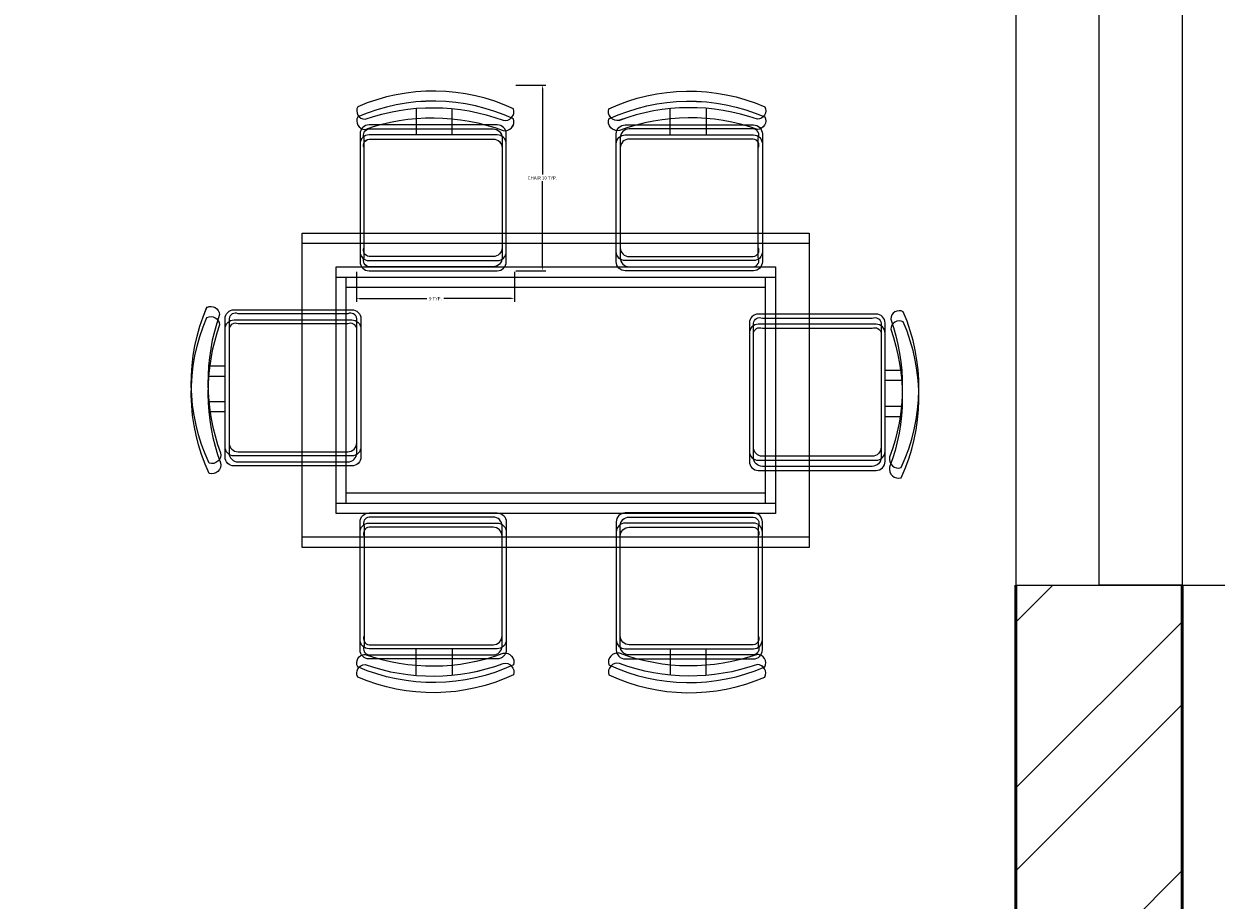
# Model space of a CAD drawing. Units: inches. Extents: x 2310 to 2937, y 1113 to 2410.
# Tile 14 of 23: x 2761 to 2826, y 1893 to 1940. Entities that reach past the tile are written whole.
import ezdxf

# ---------------------------------------------------------------- set-up
doc = ezdxf.new("R2010")
doc.units = ezdxf.units.IN
for name, color, linetype, lineweight in [('A-ANNO-DIMS', 2, 'Continuous', 18), ('A-FURN', 8, 'Continuous', 18), ('A-GLAZ', 191, 'Continuous', 20), ('A-WALL', 7, 'Continuous', 50), ('A-WALL-PATT', 85, 'Continuous', 13)]:
    doc.layers.add(name, color=color, linetype=linetype, lineweight=lineweight)
doc.styles.get("Standard").update_dxf_attribs({"font": 'arial.ttf'})
doc.dimstyles.get("Standard").update_dxf_attribs({"dimtxt": 0.18, "dimasz": 0.18, "dimexe": 0.18, "dimexo": 0.0625, "dimgap": 0.09, "dimtad": 0, "dimtih": 1, "dimtoh": 1, "dimdec": 4, "dimzin": 0, "dimdsep": 46, "dimtxsty": 'Standard', "dimcen": 0.09, "dimadec": 0, "dimazin": 0, "dimtfac": 1, "dimtdec": 4, "dimtofl": 0, "dimtmove": 0, "dimatfit": 3, "dimfxl": 1, "dimtolj": 1, "dimtzin": 0, "dimarcsym": 0})

# ---------------------------------------------------------------- blocks, each defined once
blk = doc.blocks.new('WIN-60IN')
for p, q in [((4.5, 60), (0, 60)), ((0, 60), (9, 60)), ((0, 60), (0, 0)), ((4.5, 0), (4.5, 60)), ((9, 60), (9, 0)), ((0, 0), (9, 0)), ((9, 0), (4.5, 0))]:
    blk.add_line(p, q)
blk = doc.blocks.new('DINING-TABLE')
for points in [[(0, 17.017), (27.446, 17.017), (27.446, 0.549), (0, 0.549)], [(0, 17.016), (27.446, 17.016), (27.446, 0.549), (0, 0.549)], [(0, 16.468), (27.446, 16.468), (27.446, 0), (0, 0)], [(0, 16.467), (27.446, 16.467), (27.446, 0), (0, 0)], [(1.83, 15.187), (25.616, 15.187), (25.616, 2.379), (1.83, 2.379)], [(1.83, 15.187), (25.616, 15.187), (25.616, 2.379), (1.83, 2.379)], [(1.83, 14.638), (25.616, 14.638), (25.616, 1.83), (1.83, 1.83)], [(1.83, 14.638), (25.616, 14.638), (25.616, 1.83), (1.83, 1.83)], [(2.379, 14.638), (25.067, 14.638), (25.067, 2.928), (2.379, 2.928)], [(2.379, 14.638), (25.067, 14.638), (25.067, 2.928), (2.379, 2.928)], [(2.379, 14.089), (25.067, 14.089), (25.067, 2.379), (2.379, 2.379)], [(2.379, 14.089), (25.067, 14.089), (25.067, 2.379), (2.379, 2.379)]]:
    blk.add_lwpolyline(points, close=True)
blk = doc.blocks.new('CHAIR-DINING-8')
for points in [[(0.47, 8.201, -0.175809), (7.946, 8.145, 0.578392), (8.512, 8.768, 0.214524), (0.074, 8.881, 0.552014), (0.47, 8.201, -0.065079)], [(0.47, 8.201, -0.175809), (7.946, 8.145, 0.578392), (8.512, 8.767, 0.214524), (0.074, 8.88, 0.552014), (0.47, 8.201, -0.065079)], [(0.47, 7.653, -0.175809), (7.946, 7.596, 0.578392), (8.512, 8.219, 0.214524), (0.074, 8.332, 0.552014), (0.47, 7.653, -0.065079)], [(0.47, 7.652, -0.175809), (7.946, 7.596, 0.578392), (8.512, 8.218, 0.214524), (0.074, 8.332, 0.552014), (0.47, 7.652, -0.065079)], [(5.191, 7.901), (5.191, 8.779, -0.064759)], [(5.191, 7.901), (5.191, 8.779, -0.064759)], [(7.629, 7.901), (0.689, 7.901, 0.414214), (0.203, 7.416), (0.203, 1.035, 0.414214), (0.689, 0.549), (7.629, 0.549, 0.414214), (8.114, 1.035), (8.114, 7.416, 0.414214), (7.629, 7.901)], [(7.629, 7.901), (0.689, 7.901, 0.414214), (0.203, 7.416), (0.203, 1.034, 0.414214), (0.689, 0.549), (7.629, 0.549, 0.414214), (8.114, 1.034), (8.114, 7.416, 0.414214), (7.629, 7.901)], [(5.191, 7.352), (5.191, 8.23, -0.064759)], [(5.191, 7.352), (5.191, 8.23, -0.064759)], [(7.629, 7.352), (0.689, 7.352, 0.414214), (0.203, 6.867), (0.203, 0.486, 0.414214), (0.689, 0), (7.629, 0, 0.414214), (8.114, 0.486), (8.114, 6.867, 0.414214), (7.629, 7.352)], [(7.629, 7.352), (0.689, 7.352, 0.414214), (0.203, 6.867), (0.203, 0.486, 0.414214), (0.689, 0), (7.629, 0, 0.414214), (8.114, 0.486), (8.114, 6.867, 0.414214), (7.629, 7.352)]]:
    blk.add_lwpolyline(points, format="xyb")
for points in [[(3.248, 8.795), (3.248, 7.901)], [(3.248, 8.795), (3.248, 7.901)], [(3.248, 8.246), (3.248, 7.352)], [(3.248, 8.246), (3.248, 7.352)]]:
    blk.add_lwpolyline(points)
for points in [[(0.692, 7.683), (7.41, 7.683, -0.414214), (7.895, 7.197), (7.895, 1.253, -0.414214), (7.41, 0.768), (0.692, 0.768, -0.512069), (0.422, 1.253), (0.422, 7.197, -0.512069)], [(0.692, 7.682), (7.41, 7.682, -0.414214), (7.895, 7.197), (7.895, 1.253, -0.414214), (7.41, 0.768), (0.692, 0.768, -0.512069), (0.422, 1.253), (0.422, 7.197, -0.512069)], [(0.692, 7.134), (7.41, 7.134, -0.414214), (7.895, 6.648), (7.895, 0.705, -0.414214), (7.41, 0.219), (0.692, 0.219, -0.512069), (0.422, 0.705), (0.422, 6.648, -0.512069)], [(0.692, 7.133), (7.41, 7.133, -0.414214), (7.895, 6.648), (7.895, 0.704, -0.414214), (7.41, 0.219), (0.692, 0.219, -0.512069), (0.422, 0.704), (0.422, 6.648, -0.512069)]]:
    blk.add_lwpolyline(points, format="xyb", close=True)
blk = doc.blocks.new('*D19')
at = {"layer": 'A-ANNO-DIMS', "color": 0, "lineweight": -2, "transparency": 16777216}
for p, q in [((2787.902, 1937.048), (2789.528, 1937.048)), ((2789.348, 1936.868), (2789.348, 1932.205)), ((2789.348, 1927.176), (2789.348, 1931.839)), ((2787.902, 1926.996), (2789.528, 1926.996))]:
    blk.add_line(p, q, dxfattribs=at)
at = {"layer": 'A-ANNO-DIMS', "color": 0, "transparency": 16777216}
for points in [[(2789.318, 1936.868), (2789.378, 1936.868), (2789.348, 1937.048)], [(2789.318, 1927.176), (2789.378, 1927.176), (2789.348, 1926.996)]]:
    blk.add_solid(points, dxfattribs=at)
at = {"layer": 'Defpoints', "color": 0, "transparency": 16777216}
for p in [(2787.84, 1937.048), (2789.348, 1937.048), (2787.84, 1926.996)]:
    blk.add_point(p, dxfattribs=at)
at = {"layer": 'A-ANNO-DIMS', "color": 0, "transparency": 16777216, "insert": (2789.348, 1932.022), "char_height": 0.18, "attachment_point": 5}
blk.add_mtext('\\A1;CHAIR 10 TYP.', dxfattribs=at)
blk = doc.blocks.new('*D20')
at = {"layer": 'A-ANNO-DIMS', "color": 0, "lineweight": -2, "transparency": 16777216}
for p, q in [((2779.275, 1926.934), (2779.275, 1925.308)), ((2787.84, 1926.934), (2787.84, 1925.308)), ((2779.455, 1925.488), (2783.099, 1925.488)), ((2787.66, 1925.488), (2784.016, 1925.488))]:
    blk.add_line(p, q, dxfattribs=at)
at = {"layer": 'A-ANNO-DIMS', "color": 0, "transparency": 16777216}
for points in [[(2779.455, 1925.518), (2779.455, 1925.458), (2779.275, 1925.488)], [(2787.66, 1925.518), (2787.66, 1925.458), (2787.84, 1925.488)]]:
    blk.add_solid(points, dxfattribs=at)
at = {"layer": 'Defpoints', "color": 0, "transparency": 16777216}
for p in [(2779.275, 1926.996), (2787.84, 1926.996), (2787.84, 1925.488)]:
    blk.add_point(p, dxfattribs=at)
at = {"layer": 'A-ANNO-DIMS', "color": 0, "transparency": 16777216, "insert": (2783.557, 1925.488), "char_height": 0.18, "attachment_point": 5}
blk.add_mtext('\\A1;9 TYP.', dxfattribs=at)
blk = doc.blocks.new('*D47')
at = {"layer": 'A-ANNO-DIMS', "color": 0, "lineweight": -2, "transparency": 16777216}
for p, q in [((2824.048, 1909.978), (2858.016, 1909.978)), ((2857.836, 1909.798), (2857.836, 1882.256)), ((2857.836, 1854.35), (2857.836, 1881.893)), ((2824.048, 1854.17), (2858.016, 1854.17))]:
    blk.add_line(p, q, dxfattribs=at)
at = {"layer": 'A-ANNO-DIMS', "color": 0, "transparency": 16777216}
for points in [[(2857.806, 1909.798), (2857.866, 1909.798), (2857.836, 1909.978)], [(2857.806, 1854.35), (2857.866, 1854.35), (2857.836, 1854.17)]]:
    blk.add_solid(points, dxfattribs=at)
at = {"layer": 'Defpoints', "color": 0, "transparency": 16777216}
for p in [(2823.986, 1909.978), (2857.836, 1909.978), (2823.986, 1854.17)]:
    blk.add_point(p, dxfattribs=at)
at = {"layer": 'A-ANNO-DIMS', "color": 0, "transparency": 16777216, "insert": (2857.836, 1882.074), "char_height": 0.18, "attachment_point": 5}
blk.add_mtext('\\A1;55.81', dxfattribs=at)

msp = doc.modelspace()

# ---------------------------------------------------------------- hatches: boundary and pattern name
at = {"layer": 'A-WALL-PATT'}
h = msp.add_hatch(dxfattribs=at)
h.set_pattern_fill('ANSI32', color=256)
h.paths.add_polyline_path([(2639.1394, 2356.5139), (2563.662, 2356.5139), (2563.662, 2347.5139), (2606.9859, 2347.5139), (2606.9859, 2210.5139), (2514.2692, 2210.5139), (2514.2692, 2206.0139), (2606.9859, 2206.0139), (2606.9859, 2098.0139), (2602.689, 2098.0139), (2602.689, 2093.5139), (2615.5262, 2093.5139), (2615.5262, 2095.7639), (2615.5262, 2098.0139), (2611.4859, 2098.0139), (2611.4859, 2206.0139), (2703.9391, 2206.0139), (2703.9391, 2208.2639), (2703.9391, 2210.5139), (2611.4859, 2210.5139), (2611.4859, 2347.5139), (2639.1394, 2347.5139)])
h.paths.add_polyline_path([(2823.9859, 2356.5139), (2699.1394, 2356.5139), (2699.1394, 2347.5139), (2738.4859, 2347.5139), (2738.4859, 2343.9266), (2742.9859, 2343.9266), (2742.9859, 2347.5139), (2814.9859, 2347.5139), (2814.9859, 2336.76), (2823.9859, 2336.76)])
h.paths.add_polyline_path([(2823.9859, 2312.76), (2814.9859, 2312.76), (2814.9859, 2299.5139), (2742.9859, 2299.5139), (2742.9859, 2323.0159), (2740.7359, 2323.0159), (2738.4859, 2323.0159), (2738.4859, 2210.5139), (2734.5483, 2210.5139), (2734.5483, 2206.0139), (2746.8769, 2206.0139), (2746.8769, 2208.2639), (2746.8769, 2210.5139), (2742.9859, 2210.5139), (2742.9859, 2295.0139), (2814.9859, 2295.0139), (2814.9859, 2269.8977), (2823.9859, 2269.8977)])
h.paths.add_polyline_path([(2823.9859, 2210.5139), (2823.9859, 2233.8977), (2819.4859, 2233.8977), (2814.9859, 2233.8977), (2814.9859, 2210.5139), (2769.9745, 2210.5139), (2769.9745, 2206.0139), (2814.9859, 2206.0139), (2814.9859, 2178.3027), (2823.9859, 2178.3027)])
h.paths.add_polyline_path([(2823.9859, 2118.3027), (2819.4859, 2118.3027), (2814.9859, 2118.3027), (2814.9859, 2098.0139), (2647.0333, 2098.0139), (2647.0333, 2093.5139), (2814.9859, 2093.5139), (2814.9859, 1999.5139), (2650.6052, 1999.5139), (2650.6052, 1995.0139), (2814.9859, 1995.0139), (2814.9859, 1969.9784), (2823.9859, 1969.9784)])
h.paths.add_polyline_path([(2403.4859, 2093.5139), (2569.9888, 2093.5139), (2569.9888, 2095.7639), (2569.9888, 2098.0139), (2403.4859, 2098.0139), (2403.4859, 2131.7587), (2394.4859, 2131.7587), (2394.4859, 1967.522), (2403.4859, 1967.522), (2403.4859, 1995.0139), (2569.8903, 1995.0139), (2569.8903, 1997.2639), (2569.8903, 1999.5139), (2403.4859, 1999.5139)])
h.paths.add_polyline_path([(2503.662, 2356.5139), (2394.4859, 2356.5139), (2394.4859, 2337.9231), (2398.9859, 2337.9231), (2403.4859, 2337.9231), (2403.4859, 2347.5139), (2475.4859, 2347.5139), (2475.4859, 2343.0384), (2479.9859, 2343.0384), (2479.9859, 2347.5139), (2503.662, 2347.5139)])
h.paths.add_polyline_path([(2498.3065, 1745.5139), (2479.9859, 1745.5139), (2479.9859, 1749.1663), (2477.7359, 1749.1663), (2475.4859, 1749.1663), (2475.4859, 1745.5139), (2403.4859, 1745.5139), (2403.4859, 1753.6409), (2398.9859, 1753.6409), (2394.4859, 1753.6409), (2394.4859, 1736.5139), (2498.3065, 1736.5139), (2498.3065, 1741.0139)])
h.paths.add_polyline_path([(2479.9859, 1882.5139), (2483.9367, 1882.5139), (2483.9367, 1887.0139), (2471.5501, 1887.0139), (2471.5501, 1885.1969), (2471.5501, 1882.5139), (2475.4859, 1882.5139), (2475.4859, 1798.0139), (2403.4859, 1798.0139), (2403.4859, 1828.0433), (2402.2852, 1828.0433), (2394.4859, 1828.0433), (2394.4859, 1777.6409), (2403.4859, 1777.6409), (2403.4859, 1793.5139), (2475.4859, 1793.5139), (2475.4859, 1769.1696), (2479.9859, 1769.1696)])
h.paths.add_polyline_path([(2403.4859, 1907.522), (2398.9859, 1907.522), (2394.4859, 1907.522), (2394.4859, 1864.0433), (2403.4859, 1864.0433), (2403.4859, 1882.5139), (2448.9325, 1882.5139), (2448.9325, 1884.7639), (2448.9325, 1887.0139), (2403.4859, 1887.0139)])
h.paths.add_polyline_path([(2702.2061, 1887.0139), (2611.4859, 1887.0139), (2611.4859, 1995.0139), (2615.6132, 1995.0139), (2615.6132, 1999.5139), (2602.4798, 1999.5139), (2602.4798, 1997.2639), (2602.4798, 1995.0139), (2606.9859, 1995.0139), (2606.9859, 1887.0139), (2516.2443, 1887.0139), (2516.2443, 1884.7639), (2516.2443, 1882.5139), (2606.9859, 1882.5139), (2606.9859, 1745.5139), (2558.3065, 1745.5139), (2558.3065, 1736.5139), (2638.8921, 1736.5139), (2638.8921, 1741.0139), (2638.8921, 1745.5139), (2611.4859, 1745.5139), (2611.4859, 1882.5139), (2702.2061, 1882.5139)])
h.paths.add_polyline_path([(2823.9859, 1909.9784), (2819.4859, 1909.9784), (2814.9859, 1909.9784), (2814.9859, 1887.0139), (2769.144, 1887.0139), (2769.144, 1884.7639), (2769.144, 1882.5139), (2814.9859, 1882.5139), (2814.9859, 1854.1704), (2823.9859, 1854.1704)])
h.paths.add_polyline_path([(2823.9859, 1818.1704), (2819.4859, 1818.1704), (2814.9859, 1818.1704), (2814.9859, 1798.0139), (2742.9859, 1798.0139), (2742.9859, 1882.5139), (2746.805, 1882.5139), (2746.805, 1887.0139), (2733.7334, 1887.0139), (2733.7334, 1884.7639), (2733.7334, 1882.5139), (2738.4859, 1882.5139), (2738.4859, 1771.1728), (2740.7359, 1771.1728), (2742.9859, 1771.1728), (2742.9859, 1793.5139), (2814.9859, 1793.5139), (2814.9859, 1783.6684), (2823.9859, 1783.6684)])
h.paths.add_polyline_path([(2823.9859, 1759.6684), (2814.9859, 1759.6684), (2814.9859, 1745.5139), (2742.9859, 1745.5139), (2742.9859, 1748.9831), (2740.7359, 1748.9831), (2738.4859, 1748.9831), (2738.4859, 1745.5139), (2698.8921, 1745.5139), (2698.8921, 1736.5139), (2823.9859, 1736.5139)])

# ---------------------------------------------------------------- linework, layer by layer
at = {"layer": 'A-FURN'}
for points in [[(2793.5138, 1935.1411, -0.5783921), (2792.9475, 1935.7638, -0.2145244), (2801.3857, 1935.877, -0.552014), (2800.9892, 1935.1977, 0.1758092), (2793.5138, 1935.1411)], [(2793.5138, 1935.1411, -0.5783921), (2792.9475, 1935.7638, -0.2145244), (2801.3857, 1935.877, -0.552014), (2800.9892, 1935.1977, 0.1758092), (2793.5138, 1935.1411)], [(2793.5138, 1935.1408, -0.5783921), (2792.9475, 1935.7635, -0.2145244), (2801.3857, 1935.8767, -0.552014), (2800.9893, 1935.1974, 0.1758092), (2793.5138, 1935.1408)], [(2793.5138, 1935.1408, -0.5783921), (2792.9475, 1935.7635, -0.2145244), (2801.3857, 1935.8767, -0.552014), (2800.9893, 1935.1974, 0.1758092), (2793.5138, 1935.1408)], [(2793.5138, 1934.5921, -0.5783921), (2792.9475, 1935.2148, -0.2145244), (2801.3857, 1935.3281, -0.552014), (2800.9892, 1934.6487, 0.1758092), (2793.5138, 1934.5921)], [(2793.5138, 1934.5921, -0.5783921), (2792.9475, 1935.2148, -0.2145244), (2801.3857, 1935.3281, -0.552014), (2800.9892, 1934.6487, 0.1758092), (2793.5138, 1934.5921)], [(2793.5138, 1934.5918, -0.5783921), (2792.9475, 1935.2146, -0.2145244), (2801.3857, 1935.3278, -0.552014), (2800.9893, 1934.6485, 0.1758092), (2793.5138, 1934.5918)], [(2793.5138, 1934.5918, -0.5783921), (2792.9475, 1935.2146, -0.2145244), (2801.3857, 1935.3278, -0.552014), (2800.9893, 1934.6485, 0.1758092), (2793.5138, 1934.5918)], [(2796.2686, 1934.8976), (2796.2686, 1935.7753, 0.0647586)], [(2796.2686, 1934.8976), (2796.2686, 1935.7753, 0.0647586)], [(2796.2686, 1934.8973), (2796.2686, 1935.775, 0.0647586)], [(2796.2686, 1934.8973), (2796.2686, 1935.775, 0.0647586)], [(2800.7709, 1934.8976, -0.4142136), (2801.2564, 1934.4121), (2801.2564, 1928.031, -0.4142136), (2800.7709, 1927.5454), (2793.831, 1927.5454, -0.4142136), (2793.3454, 1928.031), (2793.3454, 1934.4121, -0.4142136), (2793.831, 1934.8976), (2800.7709, 1934.8976)], [(2800.7709, 1934.8976, -0.4142136), (2801.2564, 1934.4121), (2801.2564, 1928.031, -0.4142136), (2800.7709, 1927.5454), (2793.831, 1927.5454, -0.4142136), (2793.3454, 1928.031), (2793.3454, 1934.4121, -0.4142136), (2793.831, 1934.8976), (2800.7709, 1934.8976)], [(2800.7709, 1934.8973, -0.4142136), (2801.2564, 1934.4118), (2801.2564, 1928.0307, -0.4142136), (2800.7709, 1927.5451), (2793.831, 1927.5451, -0.4142136), (2793.3454, 1928.0307), (2793.3454, 1934.4118, -0.4142136), (2793.831, 1934.8973), (2800.7709, 1934.8973)], [(2800.7709, 1934.8973, -0.4142136), (2801.2564, 1934.4118), (2801.2564, 1928.0307, -0.4142136), (2800.7709, 1927.5451), (2793.831, 1927.5451, -0.4142136), (2793.3454, 1928.0307), (2793.3454, 1934.4118, -0.4142136), (2793.831, 1934.8973), (2800.7709, 1934.8973)], [(2796.2686, 1934.3487), (2796.2686, 1935.2264, 0.0647586)], [(2796.2686, 1934.3487), (2796.2686, 1935.2264, 0.0647586)], [(2796.2686, 1934.3484), (2796.2686, 1935.2261, 0.0647586)], [(2796.2686, 1934.3484), (2796.2686, 1935.2261, 0.0647586)], [(2800.7709, 1934.3487, -0.4142136), (2801.2564, 1933.8632), (2801.2564, 1927.482, -0.4142136), (2800.7709, 1926.9965), (2793.831, 1926.9965, -0.4142136), (2793.3454, 1927.482), (2793.3454, 1933.8632, -0.4142136), (2793.831, 1934.3487), (2800.7709, 1934.3487)], [(2800.7709, 1934.3487, -0.4142136), (2801.2564, 1933.8632), (2801.2564, 1927.482, -0.4142136), (2800.7709, 1926.9965), (2793.831, 1926.9965, -0.4142136), (2793.3454, 1927.482), (2793.3454, 1933.8632, -0.4142136), (2793.831, 1934.3487), (2800.7709, 1934.3487)], [(2800.7709, 1934.3484, -0.4142136), (2801.2564, 1933.8629), (2801.2564, 1927.4818, -0.4142136), (2800.7709, 1926.9962), (2793.831, 1926.9962, -0.4142136), (2793.3454, 1927.4818), (2793.3454, 1933.8629, -0.4142136), (2793.831, 1934.3484), (2800.7709, 1934.3484)], [(2800.7709, 1934.3484, -0.4142136), (2801.2564, 1933.8629), (2801.2564, 1927.4818, -0.4142136), (2800.7709, 1926.9962), (2793.831, 1926.9962, -0.4142136), (2793.3454, 1927.4818), (2793.3454, 1933.8629, -0.4142136), (2793.831, 1934.3484), (2800.7709, 1934.3484)], [(2771.9243, 1917.1456, -0.5783921), (2771.3016, 1916.5793, -0.2145244), (2771.1883, 1925.0175, -0.552014), (2771.8677, 1924.6211, 0.1758094), (2771.9243, 1917.1456)], [(2771.9243, 1917.1456, -0.5783921), (2771.3016, 1916.5793, -0.2145244), (2771.1883, 1925.0175, -0.552014), (2771.8677, 1924.6211, 0.1758094), (2771.9243, 1917.1456)], [(2771.9243, 1917.1453, -0.5783921), (2771.3016, 1916.579, -0.2145244), (2771.1883, 1925.0172, -0.552014), (2771.8677, 1924.6208, 0.1758094), (2771.9243, 1917.1453)], [(2771.9243, 1917.1453, -0.5783921), (2771.3016, 1916.579, -0.2145244), (2771.1883, 1925.0172, -0.552014), (2771.8677, 1924.6208, 0.1758094), (2771.9243, 1917.1453)], [(2771.9243, 1916.5967, -0.5783921), (2771.3016, 1916.0304, -0.2145244), (2771.1883, 1924.4686, -0.552014), (2771.8677, 1924.0721, 0.1758094), (2771.9243, 1916.5967)], [(2771.9243, 1916.5967, -0.5783921), (2771.3016, 1916.0304, -0.2145244), (2771.1883, 1924.4686, -0.552014), (2771.8677, 1924.0721, 0.1758094), (2771.9243, 1916.5967)], [(2771.9243, 1916.5964, -0.5783921), (2771.3016, 1916.0301, -0.2145244), (2771.1883, 1924.4683, -0.552014), (2771.8677, 1924.0718, 0.1758094), (2771.9243, 1916.5964)], [(2771.9243, 1916.5964, -0.5783921), (2771.3016, 1916.0301, -0.2145244), (2771.1883, 1924.4683, -0.552014), (2771.8677, 1924.0718, 0.1758094), (2771.9243, 1916.5964)], [(2772.1677, 1924.4027, -0.4142136), (2772.6532, 1924.8882), (2779.0344, 1924.8882, -0.4142136), (2779.5199, 1924.4027), (2779.5199, 1917.4628, -0.4142136), (2779.0344, 1916.9772), (2772.6532, 1916.9772, -0.4142136), (2772.1677, 1917.4628), (2772.1677, 1924.4027)], [(2772.1677, 1924.4027, -0.4142136), (2772.6532, 1924.8882), (2779.0344, 1924.8882, -0.4142136), (2779.5199, 1924.4027), (2779.5199, 1917.4628, -0.4142136), (2779.0344, 1916.9772), (2772.6532, 1916.9772, -0.4142136), (2772.1677, 1917.4628), (2772.1677, 1924.4027)], [(2772.1677, 1924.4024, -0.4142136), (2772.6532, 1924.8879), (2779.0344, 1924.8879, -0.4142136), (2779.5199, 1924.4024), (2779.5199, 1917.4625, -0.4142136), (2779.0344, 1916.9769), (2772.6532, 1916.9769, -0.4142136), (2772.1677, 1917.4625), (2772.1677, 1924.4024)], [(2772.1677, 1924.4024, -0.4142136), (2772.6532, 1924.8879), (2779.0344, 1924.8879, -0.4142136), (2779.5199, 1924.4024), (2779.5199, 1917.4625, -0.4142136), (2779.0344, 1916.9769), (2772.6532, 1916.9769, -0.4142136), (2772.1677, 1917.4625), (2772.1677, 1924.4024)], [(2772.1677, 1923.8538, -0.4142136), (2772.6532, 1924.3393), (2779.0344, 1924.3393, -0.4142136), (2779.5199, 1923.8538), (2779.5199, 1916.9138, -0.4142136), (2779.0344, 1916.4283), (2772.6532, 1916.4283, -0.4142136), (2772.1677, 1916.9138), (2772.1677, 1923.8538)], [(2772.1677, 1923.8538, -0.4142136), (2772.6532, 1924.3393), (2779.0344, 1924.3393, -0.4142136), (2779.5199, 1923.8538), (2779.5199, 1916.9138, -0.4142136), (2779.0344, 1916.4283), (2772.6532, 1916.4283, -0.4142136), (2772.1677, 1916.9138), (2772.1677, 1923.8538)], [(2772.1677, 1923.8535, -0.4142136), (2772.6532, 1924.339), (2779.0344, 1924.339, -0.4142136), (2779.5199, 1923.8535), (2779.5199, 1916.9136, -0.4142136), (2779.0344, 1916.428), (2772.6532, 1916.428, -0.4142136), (2772.1677, 1916.9136), (2772.1677, 1923.8535)], [(2772.1677, 1923.8535, -0.4142136), (2772.6532, 1924.339), (2779.0344, 1924.339, -0.4142136), (2779.5199, 1923.8535), (2779.5199, 1916.9136, -0.4142136), (2779.0344, 1916.428), (2772.6532, 1916.428, -0.4142136), (2772.1677, 1916.9136), (2772.1677, 1923.8535)], [(2807.9051, 1924.165, 0.4142136), (2807.4196, 1924.6506), (2801.0385, 1924.6506, 0.4142136), (2800.553, 1924.165), (2800.553, 1917.2251, 0.4142136), (2801.0385, 1916.7396), (2807.4196, 1916.7396, 0.4142136), (2807.9051, 1917.2251), (2807.9051, 1924.165)], [(2807.9051, 1924.165, 0.4142136), (2807.4196, 1924.6506), (2801.0385, 1924.6506, 0.4142136), (2800.553, 1924.165), (2800.553, 1917.2251, 0.4142136), (2801.0385, 1916.7396), (2807.4196, 1916.7396, 0.4142136), (2807.9051, 1917.2251), (2807.9051, 1924.165)], [(2807.9052, 1924.1647, 0.4142136), (2807.4196, 1924.6503), (2801.0385, 1924.6503, 0.4142136), (2800.553, 1924.1647), (2800.553, 1917.2248, 0.4142136), (2801.0385, 1916.7393), (2807.4196, 1916.7393, 0.4142136), (2807.9052, 1917.2248), (2807.9052, 1924.1647)], [(2807.9052, 1924.1647, 0.4142136), (2807.4196, 1924.6503), (2801.0385, 1924.6503, 0.4142136), (2800.553, 1924.1647), (2800.553, 1917.2248, 0.4142136), (2801.0385, 1916.7393), (2807.4196, 1916.7393, 0.4142136), (2807.9052, 1917.2248), (2807.9052, 1924.1647)], [(2808.2052, 1924.3834, -0.1758092), (2808.1486, 1916.9079, 0.5783921), (2808.7713, 1916.3416, 0.2145244), (2808.8845, 1924.7798, 0.552014), (2808.2052, 1924.3834, -0.065079)], [(2808.2052, 1924.3834, -0.1758092), (2808.1486, 1916.9079, 0.5783921), (2808.7713, 1916.3416, 0.2145244), (2808.8845, 1924.7798, 0.552014), (2808.2052, 1924.3834, -0.065079)], [(2808.2052, 1924.3831, -0.1758092), (2808.1486, 1916.9076, 0.5783921), (2808.7713, 1916.3413, 0.2145244), (2808.8845, 1924.7795, 0.552014), (2808.2052, 1924.3831, -0.065079)], [(2808.2052, 1924.3831, -0.1758092), (2808.1486, 1916.9076, 0.5783921), (2808.7713, 1916.3413, 0.2145244), (2808.8845, 1924.7795, 0.552014), (2808.2052, 1924.3831, -0.065079)], [(2808.2052, 1923.8345, -0.1758092), (2808.1486, 1916.359, 0.5783921), (2808.7713, 1915.7927, 0.2145244), (2808.8845, 1924.2309, 0.552014), (2808.2052, 1923.8345, -0.065079)], [(2808.2052, 1923.8345, -0.1758092), (2808.1486, 1916.359, 0.5783921), (2808.7713, 1915.7927, 0.2145244), (2808.8845, 1924.2309, 0.552014), (2808.2052, 1923.8345, -0.065079)], [(2808.2052, 1923.8342, -0.1758092), (2808.1486, 1916.3587, 0.5783921), (2808.7713, 1915.7924, 0.2145244), (2808.8845, 1924.2306, 0.552014), (2808.2052, 1923.8342, -0.065079)], [(2808.2052, 1923.8342, -0.1758092), (2808.1486, 1916.3587, 0.5783921), (2808.7713, 1915.7924, 0.2145244), (2808.8845, 1924.2306, 0.552014), (2808.2052, 1923.8342, -0.065079)], [(2807.9051, 1923.6161, 0.4142136), (2807.4196, 1924.1016), (2801.0385, 1924.1016, 0.4142136), (2800.553, 1923.6161), (2800.553, 1916.6762, 0.4142136), (2801.0385, 1916.1906), (2807.4196, 1916.1906, 0.4142136), (2807.9051, 1916.6762), (2807.9051, 1923.6161)], [(2807.9051, 1923.6161, 0.4142136), (2807.4196, 1924.1016), (2801.0385, 1924.1016, 0.4142136), (2800.553, 1923.6161), (2800.553, 1916.6762, 0.4142136), (2801.0385, 1916.1906), (2807.4196, 1916.1906, 0.4142136), (2807.9051, 1916.6762), (2807.9051, 1923.6161)], [(2807.9052, 1923.6158, 0.4142136), (2807.4196, 1924.1014), (2801.0385, 1924.1014, 0.4142136), (2800.553, 1923.6158), (2800.553, 1916.6759, 0.4142136), (2801.0385, 1916.1904), (2807.4196, 1916.1904, 0.4142136), (2807.9052, 1916.6759), (2807.9052, 1923.6158)], [(2807.9052, 1923.6158, 0.4142136), (2807.4196, 1924.1014), (2801.0385, 1924.1014, 0.4142136), (2800.553, 1923.6158), (2800.553, 1916.6759, 0.4142136), (2801.0385, 1916.1904), (2807.4196, 1916.1904, 0.4142136), (2807.9052, 1916.6759), (2807.9052, 1923.6158)], [(2772.1677, 1919.9004), (2771.29, 1919.9004, 0.0647586)], [(2772.1677, 1919.9004), (2771.29, 1919.9004, 0.0647586)], [(2772.1677, 1919.9001), (2771.29, 1919.9001, 0.0647586)], [(2772.1677, 1919.9001), (2771.29, 1919.9001, 0.0647586)], [(2772.1677, 1919.3515), (2771.29, 1919.3515, 0.0647586)], [(2772.1677, 1919.3515), (2771.29, 1919.3515, 0.0647586)], [(2772.1677, 1919.3512), (2771.29, 1919.3512, 0.0647586)], [(2772.1677, 1919.3512), (2771.29, 1919.3512, 0.0647586)], [(2807.9051, 1919.6627), (2808.7828, 1919.6627, -0.0647586)], [(2807.9051, 1919.6627), (2808.7828, 1919.6627, -0.0647586)], [(2807.9051, 1919.1138), (2808.7828, 1919.1138, -0.0647586)], [(2807.9051, 1919.1138), (2808.7828, 1919.1138, -0.0647586)], [(2807.9052, 1919.6625), (2808.7829, 1919.6625, -0.0647586)], [(2807.9052, 1919.6625), (2808.7829, 1919.6625, -0.0647586)], [(2807.9052, 1919.1135), (2808.7829, 1919.1135, -0.0647586)], [(2807.9052, 1919.1135), (2808.7829, 1919.1135, -0.0647586)], [(2786.9033, 1906.5319), (2779.9634, 1906.5319, -0.4142136), (2779.4778, 1907.0174), (2779.4778, 1913.3986, -0.4142136), (2779.9634, 1913.8841), (2786.9033, 1913.8841, -0.4142136), (2787.3888, 1913.3986), (2787.3888, 1907.0174, -0.4142136), (2786.9033, 1906.5319)], [(2786.9033, 1906.5319), (2779.9634, 1906.5319, -0.4142136), (2779.4778, 1907.0174), (2779.4778, 1913.3986, -0.4142136), (2779.9634, 1913.8841), (2786.9033, 1913.8841, -0.4142136), (2787.3888, 1913.3986), (2787.3888, 1907.0174, -0.4142136), (2786.9033, 1906.5319)], [(2786.9033, 1906.5316), (2779.9634, 1906.5316, -0.4142136), (2779.4778, 1907.0171), (2779.4778, 1913.3983, -0.4142136), (2779.9634, 1913.8838), (2786.9033, 1913.8838, -0.4142136), (2787.3888, 1913.3983), (2787.3888, 1907.0171, -0.4142136), (2786.9033, 1906.5316)], [(2786.9033, 1906.5316), (2779.9634, 1906.5316, -0.4142136), (2779.4778, 1907.0171), (2779.4778, 1913.3983, -0.4142136), (2779.9634, 1913.8838), (2786.9033, 1913.8838, -0.4142136), (2787.3888, 1913.3983), (2787.3888, 1907.0171, -0.4142136), (2786.9033, 1906.5316)], [(2786.9033, 1905.983), (2779.9634, 1905.983, -0.4142136), (2779.4778, 1906.4685), (2779.4778, 1912.8496, -0.4142136), (2779.9634, 1913.3352), (2786.9033, 1913.3352, -0.4142136), (2787.3888, 1912.8496), (2787.3888, 1906.4685, -0.4142136), (2786.9033, 1905.983)], [(2786.9033, 1905.983), (2779.9634, 1905.983, -0.4142136), (2779.4778, 1906.4685), (2779.4778, 1912.8496, -0.4142136), (2779.9634, 1913.3352), (2786.9033, 1913.3352, -0.4142136), (2787.3888, 1912.8496), (2787.3888, 1906.4685, -0.4142136), (2786.9033, 1905.983)], [(2786.9033, 1905.9827), (2779.9634, 1905.9827, -0.4142136), (2779.4778, 1906.4682), (2779.4778, 1912.8494, -0.4142136), (2779.9634, 1913.3349), (2786.9033, 1913.3349, -0.4142136), (2787.3888, 1912.8494), (2787.3888, 1906.4682, -0.4142136), (2786.9033, 1905.9827)], [(2786.9033, 1905.9827), (2779.9634, 1905.9827, -0.4142136), (2779.4778, 1906.4682), (2779.4778, 1912.8494, -0.4142136), (2779.9634, 1913.3349), (2786.9033, 1913.3349, -0.4142136), (2787.3888, 1912.8494), (2787.3888, 1906.4682, -0.4142136), (2786.9033, 1905.9827)], [(2800.7709, 1906.5319, 0.4142136), (2801.2564, 1907.0174), (2801.2564, 1913.3986, 0.4142136), (2800.7709, 1913.8841), (2793.831, 1913.8841, 0.4142136), (2793.3454, 1913.3986), (2793.3454, 1907.0174, 0.4142136), (2793.831, 1906.5319), (2800.7709, 1906.5319)], [(2800.7709, 1906.5319, 0.4142136), (2801.2564, 1907.0174), (2801.2564, 1913.3986, 0.4142136), (2800.7709, 1913.8841), (2793.831, 1913.8841, 0.4142136), (2793.3454, 1913.3986), (2793.3454, 1907.0174, 0.4142136), (2793.831, 1906.5319), (2800.7709, 1906.5319)], [(2800.7709, 1906.5316, 0.4142136), (2801.2564, 1907.0171), (2801.2564, 1913.3983, 0.4142136), (2800.7709, 1913.8838), (2793.831, 1913.8838, 0.4142136), (2793.3454, 1913.3983), (2793.3454, 1907.0171, 0.4142136), (2793.831, 1906.5316), (2800.7709, 1906.5316)], [(2800.7709, 1906.5316, 0.4142136), (2801.2564, 1907.0171), (2801.2564, 1913.3983, 0.4142136), (2800.7709, 1913.8838), (2793.831, 1913.8838, 0.4142136), (2793.3454, 1913.3983), (2793.3454, 1907.0171, 0.4142136), (2793.831, 1906.5316), (2800.7709, 1906.5316)], [(2800.7709, 1905.983, 0.4142136), (2801.2564, 1906.4685), (2801.2564, 1912.8496, 0.4142136), (2800.7709, 1913.3352), (2793.831, 1913.3352, 0.4142136), (2793.3454, 1912.8496), (2793.3454, 1906.4685, 0.4142136), (2793.831, 1905.983), (2800.7709, 1905.983)], [(2800.7709, 1905.983, 0.4142136), (2801.2564, 1906.4685), (2801.2564, 1912.8496, 0.4142136), (2800.7709, 1913.3352), (2793.831, 1913.3352, 0.4142136), (2793.3454, 1912.8496), (2793.3454, 1906.4685, 0.4142136), (2793.831, 1905.983), (2800.7709, 1905.983)], [(2800.7709, 1905.9827, 0.4142136), (2801.2564, 1906.4682), (2801.2564, 1912.8494, 0.4142136), (2800.7709, 1913.3349), (2793.831, 1913.3349, 0.4142136), (2793.3454, 1912.8494), (2793.3454, 1906.4682, 0.4142136), (2793.831, 1905.9827), (2800.7709, 1905.9827)], [(2800.7709, 1905.9827, 0.4142136), (2801.2564, 1906.4682), (2801.2564, 1912.8494, 0.4142136), (2800.7709, 1913.3349), (2793.831, 1913.3349, 0.4142136), (2793.3454, 1912.8494), (2793.3454, 1906.4682, 0.4142136), (2793.831, 1905.9827), (2800.7709, 1905.9827)], [(2787.2204, 1906.2885, -0.5783921), (2787.7868, 1905.6657, -0.2145244), (2779.3486, 1905.5525, -0.552014), (2779.745, 1906.2319, 0.1758093), (2787.2204, 1906.2885)], [(2787.2204, 1906.2885, -0.5783921), (2787.7868, 1905.6657, -0.2145244), (2779.3486, 1905.5525, -0.552014), (2779.745, 1906.2319, 0.1758093), (2787.2204, 1906.2885)], [(2787.2205, 1906.2882, -0.5783921), (2787.7868, 1905.6655, -0.2145244), (2779.3486, 1905.5522, -0.552014), (2779.745, 1906.2316, 0.1758093), (2787.2205, 1906.2882)], [(2787.2205, 1906.2882, -0.5783921), (2787.7868, 1905.6655, -0.2145244), (2779.3486, 1905.5522, -0.552014), (2779.745, 1906.2316, 0.1758093), (2787.2205, 1906.2882)], [(2784.4656, 1906.5319), (2784.4656, 1905.6542, 0.0647586)], [(2784.4656, 1906.5319), (2784.4656, 1905.6542, 0.0647586)], [(2784.4657, 1906.5316), (2784.4657, 1905.6539, 0.0647586)], [(2784.4657, 1906.5316), (2784.4657, 1905.6539, 0.0647586)], [(2800.9892, 1906.2319, -0.1758093), (2793.5138, 1906.2885, 0.5783921), (2792.9475, 1905.6657, 0.2145244), (2801.3857, 1905.5525, 0.552014), (2800.9892, 1906.2319, -0.065079)], [(2800.9892, 1906.2319, -0.1758093), (2793.5138, 1906.2885, 0.5783921), (2792.9475, 1905.6657, 0.2145244), (2801.3857, 1905.5525, 0.552014), (2800.9892, 1906.2319, -0.065079)], [(2800.9893, 1906.2316, -0.1758093), (2793.5138, 1906.2882, 0.5783921), (2792.9475, 1905.6655, 0.2145244), (2801.3857, 1905.5522, 0.552014), (2800.9893, 1906.2316, -0.065079)], [(2800.9893, 1906.2316, -0.1758093), (2793.5138, 1906.2882, 0.5783921), (2792.9475, 1905.6655, 0.2145244), (2801.3857, 1905.5522, 0.552014), (2800.9893, 1906.2316, -0.065079)], [(2796.2686, 1906.5319), (2796.2686, 1905.6542, -0.0647586)], [(2796.2686, 1906.5319), (2796.2686, 1905.6542, -0.0647586)], [(2796.2686, 1906.5316), (2796.2686, 1905.6539, -0.0647586)], [(2796.2686, 1906.5316), (2796.2686, 1905.6539, -0.0647586)], [(2787.2204, 1905.7395, -0.5783921), (2787.7868, 1905.1168, -0.2145244), (2779.3486, 1905.0036, -0.552014), (2779.745, 1905.6829, 0.1758093), (2787.2204, 1905.7395)], [(2787.2204, 1905.7395, -0.5783921), (2787.7868, 1905.1168, -0.2145244), (2779.3486, 1905.0036, -0.552014), (2779.745, 1905.6829, 0.1758093), (2787.2204, 1905.7395)], [(2787.2205, 1905.7393, -0.5783921), (2787.7868, 1905.1165, -0.2145244), (2779.3486, 1905.0033, -0.552014), (2779.745, 1905.6827, 0.1758093), (2787.2205, 1905.7393)], [(2787.2205, 1905.7393, -0.5783921), (2787.7868, 1905.1165, -0.2145244), (2779.3486, 1905.0033, -0.552014), (2779.745, 1905.6827, 0.1758093), (2787.2205, 1905.7393)], [(2784.4656, 1905.983), (2784.4656, 1905.1053, 0.0647586)], [(2784.4656, 1905.983), (2784.4656, 1905.1053, 0.0647586)], [(2784.4657, 1905.9827), (2784.4657, 1905.105, 0.0647586)], [(2784.4657, 1905.9827), (2784.4657, 1905.105, 0.0647586)], [(2800.9892, 1905.6829, -0.1758093), (2793.5138, 1905.7395, 0.5783921), (2792.9475, 1905.1168, 0.2145244), (2801.3857, 1905.0036, 0.552014), (2800.9892, 1905.6829, -0.065079)], [(2800.9892, 1905.6829, -0.1758093), (2793.5138, 1905.7395, 0.5783921), (2792.9475, 1905.1168, 0.2145244), (2801.3857, 1905.0036, 0.552014), (2800.9892, 1905.6829, -0.065079)], [(2800.9893, 1905.6827, -0.1758093), (2793.5138, 1905.7393, 0.5783921), (2792.9475, 1905.1165, 0.2145244), (2801.3857, 1905.0033, 0.552014), (2800.9893, 1905.6827, -0.065079)], [(2800.9893, 1905.6827, -0.1758093), (2793.5138, 1905.7393, 0.5783921), (2792.9475, 1905.1165, 0.2145244), (2801.3857, 1905.0033, 0.552014), (2800.9893, 1905.6827, -0.065079)], [(2796.2686, 1905.983), (2796.2686, 1905.1053, -0.0647586)], [(2796.2686, 1905.983), (2796.2686, 1905.1053, -0.0647586)], [(2796.2686, 1905.9827), (2796.2686, 1905.105, -0.0647586)], [(2796.2686, 1905.9827), (2796.2686, 1905.105, -0.0647586)]]:
    msp.add_lwpolyline(points, format="xyb", dxfattribs=at)
for points in [[(2798.2112, 1935.7913), (2798.2112, 1934.8976)], [(2798.2112, 1935.7913), (2798.2112, 1934.8976)], [(2798.2112, 1935.791), (2798.2112, 1934.8973)], [(2798.2112, 1935.791), (2798.2112, 1934.8973)], [(2798.2112, 1935.2424), (2798.2112, 1934.3487)], [(2798.2112, 1935.2424), (2798.2112, 1934.3487)], [(2798.2112, 1935.2421), (2798.2112, 1934.3484)], [(2798.2112, 1935.2421), (2798.2112, 1934.3484)], [(2771.274, 1921.843), (2772.1677, 1921.843)], [(2771.274, 1921.843), (2772.1677, 1921.843)], [(2771.2741, 1921.8427), (2772.1677, 1921.8427)], [(2771.2741, 1921.8427), (2772.1677, 1921.8427)], [(2771.274, 1921.2941), (2772.1677, 1921.2941)], [(2771.274, 1921.2941), (2772.1677, 1921.2941)], [(2771.2741, 1921.2938), (2772.1677, 1921.2938)], [(2771.2741, 1921.2938), (2772.1677, 1921.2938)], [(2808.7988, 1921.6053), (2807.9051, 1921.6053)], [(2808.7988, 1921.6053), (2807.9051, 1921.6053)], [(2808.7988, 1921.0564), (2807.9051, 1921.0564)], [(2808.7988, 1921.0564), (2807.9051, 1921.0564)], [(2808.7988, 1921.605), (2807.9052, 1921.605)], [(2808.7988, 1921.605), (2807.9052, 1921.605)], [(2808.7988, 1921.0561), (2807.9052, 1921.0561)], [(2808.7988, 1921.0561), (2807.9052, 1921.0561)], [(2782.523, 1905.6382), (2782.523, 1906.5319)], [(2782.523, 1905.6382), (2782.523, 1906.5319)], [(2782.5231, 1905.638), (2782.5231, 1906.5316)], [(2782.5231, 1905.638), (2782.5231, 1906.5316)], [(2798.2112, 1905.6382), (2798.2112, 1906.5319)], [(2798.2112, 1905.6382), (2798.2112, 1906.5319)], [(2798.2112, 1905.638), (2798.2112, 1906.5316)], [(2798.2112, 1905.638), (2798.2112, 1906.5316)], [(2782.523, 1905.0893), (2782.523, 1905.983)], [(2782.523, 1905.0893), (2782.523, 1905.983)], [(2782.5231, 1905.089), (2782.5231, 1905.9827)], [(2782.5231, 1905.089), (2782.5231, 1905.9827)], [(2798.2112, 1905.0893), (2798.2112, 1905.983)], [(2798.2112, 1905.0893), (2798.2112, 1905.983)], [(2798.2112, 1905.089), (2798.2112, 1905.9827)], [(2798.2112, 1905.089), (2798.2112, 1905.9827)]]:
    msp.add_lwpolyline(points, dxfattribs=at)
for points in [[(2800.768, 1934.6789), (2794.0497, 1934.6789, 0.4142136), (2793.5642, 1934.1934), (2793.5642, 1928.2497, 0.4142136), (2794.0497, 1927.7642), (2800.768, 1927.7642, 0.5120695), (2801.0377, 1928.2497), (2801.0377, 1934.1934, 0.5120695)], [(2800.768, 1934.6789), (2794.0497, 1934.6789, 0.4142136), (2793.5642, 1934.1934), (2793.5642, 1928.2497, 0.4142136), (2794.0497, 1927.7642), (2800.768, 1927.7642, 0.5120695), (2801.0377, 1928.2497), (2801.0377, 1934.1934, 0.5120695)], [(2800.768, 1934.6786), (2794.0497, 1934.6786, 0.4142136), (2793.5642, 1934.1931), (2793.5642, 1928.2494, 0.4142136), (2794.0497, 1927.7639), (2800.768, 1927.7639, 0.5120695), (2801.0377, 1928.2494), (2801.0377, 1934.1931, 0.5120695)], [(2800.768, 1934.6786), (2794.0497, 1934.6786, 0.4142136), (2793.5642, 1934.1931), (2793.5642, 1928.2494, 0.4142136), (2794.0497, 1927.7639), (2800.768, 1927.7639, 0.5120695), (2801.0377, 1928.2494), (2801.0377, 1934.1931, 0.5120695)], [(2800.768, 1934.13), (2794.0497, 1934.13, 0.4142136), (2793.5642, 1933.6445), (2793.5642, 1927.7008, 0.4142136), (2794.0497, 1927.2153), (2800.768, 1927.2153, 0.5120695), (2801.0377, 1927.7008), (2801.0377, 1933.6445, 0.5120695)], [(2800.768, 1934.13), (2794.0497, 1934.13, 0.4142136), (2793.5642, 1933.6445), (2793.5642, 1927.7008, 0.4142136), (2794.0497, 1927.2153), (2800.768, 1927.2153, 0.5120695), (2801.0377, 1927.7008), (2801.0377, 1933.6445, 0.5120695)], [(2800.768, 1934.1297), (2794.0497, 1934.1297, 0.4142136), (2793.5642, 1933.6442), (2793.5642, 1927.7005, 0.4142136), (2794.0497, 1927.215), (2800.768, 1927.215, 0.5120695), (2801.0377, 1927.7005), (2801.0377, 1933.6442, 0.5120695)], [(2800.768, 1934.1297), (2794.0497, 1934.1297, 0.4142136), (2793.5642, 1933.6442), (2793.5642, 1927.7005, 0.4142136), (2794.0497, 1927.215), (2800.768, 1927.215, 0.5120695), (2801.0377, 1927.7005), (2801.0377, 1933.6442, 0.5120695)], [(2772.3864, 1924.3998), (2772.3864, 1917.6815, 0.4142136), (2772.8719, 1917.196), (2778.8156, 1917.196, 0.4142136), (2779.3012, 1917.6815), (2779.3012, 1924.3998, 0.5120695), (2778.8156, 1924.6695), (2772.8719, 1924.6695, 0.5120695)], [(2772.3864, 1924.3998), (2772.3864, 1917.6815, 0.4142136), (2772.8719, 1917.196), (2778.8156, 1917.196, 0.4142136), (2779.3012, 1917.6815), (2779.3012, 1924.3998, 0.5120695), (2778.8156, 1924.6695), (2772.8719, 1924.6695, 0.5120695)], [(2772.3864, 1924.3995), (2772.3864, 1917.6812, 0.4142136), (2772.872, 1917.1957), (2778.8156, 1917.1957, 0.4142136), (2779.3012, 1917.6812), (2779.3012, 1924.3995, 0.5120695), (2778.8156, 1924.6692), (2772.872, 1924.6692, 0.5120695)], [(2772.3864, 1924.3995), (2772.3864, 1917.6812, 0.4142136), (2772.872, 1917.1957), (2778.8156, 1917.1957, 0.4142136), (2779.3012, 1917.6812), (2779.3012, 1924.3995, 0.5120695), (2778.8156, 1924.6692), (2772.872, 1924.6692, 0.5120695)], [(2807.6864, 1924.1621), (2807.6864, 1917.4438, -0.4142136), (2807.2009, 1916.9583), (2801.2572, 1916.9583, -0.4142136), (2800.7717, 1917.4438), (2800.7717, 1924.1621, -0.5120695), (2801.2572, 1924.4318), (2807.2009, 1924.4318, -0.5120695)], [(2807.6864, 1924.1621), (2807.6864, 1917.4438, -0.4142136), (2807.2009, 1916.9583), (2801.2572, 1916.9583, -0.4142136), (2800.7717, 1917.4438), (2800.7717, 1924.1621, -0.5120695), (2801.2572, 1924.4318), (2807.2009, 1924.4318, -0.5120695)], [(2807.6864, 1924.1618), (2807.6864, 1917.4435, -0.4142136), (2807.2009, 1916.958), (2801.2572, 1916.958, -0.4142136), (2800.7717, 1917.4435), (2800.7717, 1924.1618, -0.5120695), (2801.2572, 1924.4315), (2807.2009, 1924.4315, -0.5120695)], [(2807.6864, 1924.1618), (2807.6864, 1917.4435, -0.4142136), (2807.2009, 1916.958), (2801.2572, 1916.958, -0.4142136), (2800.7717, 1917.4435), (2800.7717, 1924.1618, -0.5120695), (2801.2572, 1924.4315), (2807.2009, 1924.4315, -0.5120695)], [(2772.3864, 1923.8508), (2772.3864, 1917.1326, 0.4142136), (2772.8719, 1916.6471), (2778.8156, 1916.6471, 0.4142136), (2779.3012, 1917.1326), (2779.3012, 1923.8508, 0.5120695), (2778.8156, 1924.1206), (2772.8719, 1924.1206, 0.5120695)], [(2772.3864, 1923.8508), (2772.3864, 1917.1326, 0.4142136), (2772.8719, 1916.6471), (2778.8156, 1916.6471, 0.4142136), (2779.3012, 1917.1326), (2779.3012, 1923.8508, 0.5120695), (2778.8156, 1924.1206), (2772.8719, 1924.1206, 0.5120695)], [(2772.3864, 1923.8506), (2772.3864, 1917.1323, 0.4142136), (2772.872, 1916.6468), (2778.8156, 1916.6468, 0.4142136), (2779.3012, 1917.1323), (2779.3012, 1923.8506, 0.5120695), (2778.8156, 1924.1203), (2772.872, 1924.1203, 0.5120695)], [(2772.3864, 1923.8506), (2772.3864, 1917.1323, 0.4142136), (2772.872, 1916.6468), (2778.8156, 1916.6468, 0.4142136), (2779.3012, 1917.1323), (2779.3012, 1923.8506, 0.5120695), (2778.8156, 1924.1203), (2772.872, 1924.1203, 0.5120695)], [(2807.6864, 1923.6132), (2807.6864, 1916.8949, -0.4142136), (2807.2009, 1916.4094), (2801.2572, 1916.4094, -0.4142136), (2800.7717, 1916.8949), (2800.7717, 1923.6132, -0.5120695), (2801.2572, 1923.8829), (2807.2009, 1923.8829, -0.5120695)], [(2807.6864, 1923.6132), (2807.6864, 1916.8949, -0.4142136), (2807.2009, 1916.4094), (2801.2572, 1916.4094, -0.4142136), (2800.7717, 1916.8949), (2800.7717, 1923.6132, -0.5120695), (2801.2572, 1923.8829), (2807.2009, 1923.8829, -0.5120695)], [(2807.6864, 1923.6129), (2807.6864, 1916.8946, -0.4142136), (2807.2009, 1916.4091), (2801.2572, 1916.4091, -0.4142136), (2800.7717, 1916.8946), (2800.7717, 1923.6129, -0.5120695), (2801.2572, 1923.8826), (2807.2009, 1923.8826, -0.5120695)], [(2807.6864, 1923.6129), (2807.6864, 1916.8946, -0.4142136), (2807.2009, 1916.4091), (2801.2572, 1916.4091, -0.4142136), (2800.7717, 1916.8946), (2800.7717, 1923.6129, -0.5120695), (2801.2572, 1923.8826), (2807.2009, 1923.8826, -0.5120695)], [(2779.9663, 1906.7506), (2786.6846, 1906.7506, 0.4142136), (2787.1701, 1907.2361), (2787.1701, 1913.1798, 0.4142136), (2786.6846, 1913.6653), (2779.9663, 1913.6653, 0.5120695), (2779.6966, 1913.1798), (2779.6966, 1907.2361, 0.5120695)], [(2779.9663, 1906.7506), (2786.6846, 1906.7506, 0.4142136), (2787.1701, 1907.2361), (2787.1701, 1913.1798, 0.4142136), (2786.6846, 1913.6653), (2779.9663, 1913.6653, 0.5120695), (2779.6966, 1913.1798), (2779.6966, 1907.2361, 0.5120695)], [(2779.9663, 1906.7503), (2786.6846, 1906.7503, 0.4142136), (2787.1701, 1907.2359), (2787.1701, 1913.1795, 0.4142136), (2786.6846, 1913.6651), (2779.9663, 1913.6651, 0.5120695), (2779.6966, 1913.1795), (2779.6966, 1907.2359, 0.5120695)], [(2779.9663, 1906.7503), (2786.6846, 1906.7503, 0.4142136), (2787.1701, 1907.2359), (2787.1701, 1913.1795, 0.4142136), (2786.6846, 1913.6651), (2779.9663, 1913.6651, 0.5120695), (2779.6966, 1913.1795), (2779.6966, 1907.2359, 0.5120695)], [(2800.768, 1906.7506), (2794.0497, 1906.7506, -0.4142136), (2793.5642, 1907.2361), (2793.5642, 1913.1798, -0.4142136), (2794.0497, 1913.6653), (2800.768, 1913.6653, -0.5120695), (2801.0377, 1913.1798), (2801.0377, 1907.2361, -0.5120695)], [(2800.768, 1906.7506), (2794.0497, 1906.7506, -0.4142136), (2793.5642, 1907.2361), (2793.5642, 1913.1798, -0.4142136), (2794.0497, 1913.6653), (2800.768, 1913.6653, -0.5120695), (2801.0377, 1913.1798), (2801.0377, 1907.2361, -0.5120695)], [(2800.768, 1906.7503), (2794.0497, 1906.7503, -0.4142136), (2793.5642, 1907.2359), (2793.5642, 1913.1795, -0.4142136), (2794.0497, 1913.6651), (2800.768, 1913.6651, -0.5120695), (2801.0377, 1913.1795), (2801.0377, 1907.2359, -0.5120695)], [(2800.768, 1906.7503), (2794.0497, 1906.7503, -0.4142136), (2793.5642, 1907.2359), (2793.5642, 1913.1795, -0.4142136), (2794.0497, 1913.6651), (2800.768, 1913.6651, -0.5120695), (2801.0377, 1913.1795), (2801.0377, 1907.2359, -0.5120695)], [(2779.9663, 1906.2017), (2786.6846, 1906.2017, 0.4142136), (2787.1701, 1906.6872), (2787.1701, 1912.6309, 0.4142136), (2786.6846, 1913.1164), (2779.9663, 1913.1164, 0.5120695), (2779.6966, 1912.6309), (2779.6966, 1906.6872, 0.5120695)], [(2779.9663, 1906.2017), (2786.6846, 1906.2017, 0.4142136), (2787.1701, 1906.6872), (2787.1701, 1912.6309, 0.4142136), (2786.6846, 1913.1164), (2779.9663, 1913.1164, 0.5120695), (2779.6966, 1912.6309), (2779.6966, 1906.6872, 0.5120695)], [(2779.9663, 1906.2014), (2786.6846, 1906.2014, 0.4142136), (2787.1701, 1906.6869), (2787.1701, 1912.6306, 0.4142136), (2786.6846, 1913.1161), (2779.9663, 1913.1161, 0.5120695), (2779.6966, 1912.6306), (2779.6966, 1906.6869, 0.5120695)], [(2779.9663, 1906.2014), (2786.6846, 1906.2014, 0.4142136), (2787.1701, 1906.6869), (2787.1701, 1912.6306, 0.4142136), (2786.6846, 1913.1161), (2779.9663, 1913.1161, 0.5120695), (2779.6966, 1912.6306), (2779.6966, 1906.6869, 0.5120695)], [(2800.768, 1906.2017), (2794.0497, 1906.2017, -0.4142136), (2793.5642, 1906.6872), (2793.5642, 1912.6309, -0.4142136), (2794.0497, 1913.1164), (2800.768, 1913.1164, -0.5120695), (2801.0377, 1912.6309), (2801.0377, 1906.6872, -0.5120695)], [(2800.768, 1906.2017), (2794.0497, 1906.2017, -0.4142136), (2793.5642, 1906.6872), (2793.5642, 1912.6309, -0.4142136), (2794.0497, 1913.1164), (2800.768, 1913.1164, -0.5120695), (2801.0377, 1912.6309), (2801.0377, 1906.6872, -0.5120695)], [(2800.768, 1906.2014), (2794.0497, 1906.2014, -0.4142136), (2793.5642, 1906.6869), (2793.5642, 1912.6306, -0.4142136), (2794.0497, 1913.1161), (2800.768, 1913.1161, -0.5120695), (2801.0377, 1912.6306), (2801.0377, 1906.6869, -0.5120695)], [(2800.768, 1906.2014), (2794.0497, 1906.2014, -0.4142136), (2793.5642, 1906.6869), (2793.5642, 1912.6306, -0.4142136), (2794.0497, 1913.1161), (2800.768, 1913.1161, -0.5120695), (2801.0377, 1912.6306), (2801.0377, 1906.6869, -0.5120695)]]:
    msp.add_lwpolyline(points, format="xyb", close=True, dxfattribs=at)
at = {"layer": 'A-WALL'}
for p, q in [((2814.9859, 1887.0139), (2814.9859, 1909.9784)), ((2823.9859, 1909.9784), (2823.9859, 1854.1704))]:
    msp.add_line(p, q, dxfattribs=at)

# ---------------------------------------------------------------- block references
at = {"layer": 'A-FURN'}
for name, p in [('CHAIR-DINING-8', (2779.2748, 1926.9962)), ('CHAIR-DINING-8', (2779.2748, 1926.9962)), ('DINING-TABLE', (2776.3503, 1912.02)), ('DINING-TABLE', (2776.3503, 1912.02))]:
    msp.add_blockref(name, p, dxfattribs=at)
at = {"layer": 'A-GLAZ'}
msp.add_blockref('WIN-60IN', (2814.9859, 1909.9784), dxfattribs=at)

# ---------------------------------------------------------------- dimensions: what is measured, and where the dimension line sits
at = {"layer": 'A-ANNO-DIMS'}
dim = msp.add_linear_dim(base=(2789.3476, 1937.0478), p1=(2787.8399, 1926.9962), p2=(2787.8399, 1937.0478), angle=90, text='CHAIR <> TYP.', dimstyle='Standard', override={"dimdec": 0, "dimlfac": 1, "dimrnd": 0, "dimzin": 0, "dimdsep": 46, "dimlunit": 2}, dxfattribs=at)
dim.commit()
dim.dimension.update_dxf_attribs({"geometry": '*D19', "text_midpoint": (2789.3476, 1932.022)})
dim = msp.add_linear_dim(base=(2787.8399, 1925.4885), p1=(2779.2748, 1926.9962), p2=(2787.8399, 1926.9962), text='<> TYP.', dimstyle='Standard', override={"dimdec": 0, "dimlfac": 1, "dimrnd": 0, "dimzin": 0, "dimdsep": 46, "dimlunit": 2}, dxfattribs=at)
dim.commit()
dim.dimension.update_dxf_attribs({"geometry": '*D20', "text_midpoint": (2783.5573, 1925.4885)})
dim = msp.add_linear_dim(base=(2857.8359, 1909.9784), p1=(2823.9859, 1854.1704), p2=(2823.9859, 1909.9784), angle=90, dimstyle='Standard', override={"dimdec": 2, "dimlfac": 1, "dimrnd": 0, "dimzin": 0, "dimdsep": 46, "dimlunit": 2}, dxfattribs=at)
dim.commit()
dim.dimension.update_dxf_attribs({"geometry": '*D47', "text_midpoint": (2857.8359, 1882.0744)})

doc.saveas('drawing.dxf')
